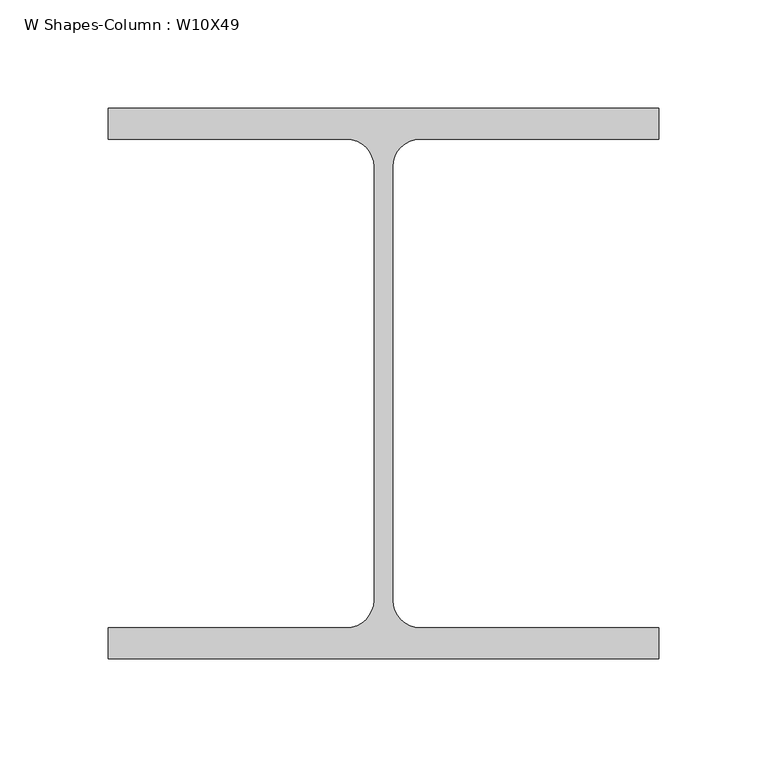
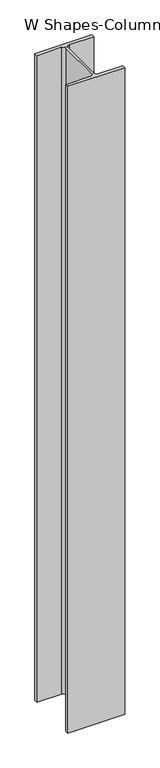
"""IFC4 building model written with IfcOpenShell, lengths in millimetres: column geometry, W Shapes-Column : W10X49."""

from ifc_helpers import new_model, si_unit, point, frame, frame_2d, origin, place, context, project, spatial, polyline, circle_curve, trimmed, segment, composite_curve, outline, extrude, source, transform, mapped, element, save


def w_shapes_column_w10x49_c7b378f5(model_context):
    return source(origin(), model_context, "Body", "SweptSolid", [
        extrude(outline(composite_curve([segment(polyline([(127.0, 127.0), (127.0, 112.776), (17.018, 112.776)]), True, "CONTINUOUS"), segment(trimmed(circle_curve(frame_2d((17.018, 100.076)), 12.7), [point((17.018, 112.776))], [point((4.318, 100.076))], True, "CARTESIAN"), True, "CONTINUOUS"), segment(polyline([(4.318, 100.076), (4.318, -100.076)]), True, "CONTINUOUS"), segment(trimmed(circle_curve(frame_2d((17.018, -100.076)), 12.7), [point((4.318, -100.076))], [point((17.018, -112.776))], True, "CARTESIAN"), True, "CONTINUOUS"), segment(polyline([(17.018, -112.776), (127.0, -112.776), (127.0, -127.0), (-127.0, -127.0), (-127.0, -112.776), (-17.018, -112.776)]), True, "CONTINUOUS"), segment(trimmed(circle_curve(frame_2d((-17.018, -100.076)), 12.7), [point((-17.018, -112.776))], [point((-4.318, -100.076))], True, "CARTESIAN"), True, "CONTINUOUS"), segment(polyline([(-4.318, -100.076), (-4.318, 100.076)]), True, "CONTINUOUS"), segment(trimmed(circle_curve(frame_2d((-17.018, 100.076)), 12.7), [point((-4.318, 100.076))], [point((-17.018, 112.776))], True, "CARTESIAN"), True, "CONTINUOUS"), segment(polyline([(-17.018, 112.776), (-127.0, 112.776), (-127.0, 127.0), (127.0, 127.0)]), True, "CONTINUOUS")], self_intersect=False)), frame((0.0, 0.0, 6096.0), z_axis=(0.0, 0.0, 1.0), x_axis=(1.0, 0.0, 0.0)), (0.0, 0.0, 1.0), 3048.0),
    ])


if __name__ == "__main__":
    model = new_model("IFC4")
    model_context = context("Model", 3, world=origin())
    ifc_project = project(units=[si_unit("LENGTHUNIT", "METRE", prefix="MILLI")], contexts=[model_context])
    site = spatial("IfcSite", under=ifc_project)
    building = spatial("IfcBuilding", under=site)
    placement = place(None, origin())
    w_shapes_column_w10x49_shape = w_shapes_column_w10x49_c7b378f5(model_context)
    element("IfcColumn", 1, ObjectType="W Shapes-Column : W10X49", at=placement, inside=building, context=model_context, shape_type="MappedRepresentation", body=[
        mapped(w_shapes_column_w10x49_shape, transform((0.0, 0.0, 0.0), x_axis=(1.0, 0.0, 0.0), y_axis=(0.0, 1.0, 0.0), z_axis=(0.0, 0.0, 1.0))),
    ])
    save(model, "model.ifc")

# Revit data of these elements
# Type "W Shapes-Column : W10X49"
#   Section Name Key = "W10x49"
#   Assembly Code = "B10"
#   Width = 10.000"
#   Web Thickness = 0.340"
#   Web Fillet = 0.500"
#   Warping Constant = 2070.00 in⁶
#   Torsional Moment of Inertia = 1.39 in⁴
#   Section Area = 14.40 in²
#   Plastic Modulus weak axis = 28.30 in³
#   Plastic Modulus strong axis = 60.40 in³
#   Perimeter = 58.50 ft²/ft
#   Nominal Weight = 49.00 lbf/ft
#   Moment of Inertia weak axis = 93.40 in⁴
#   Moment of Inertia strong axis = 272.00 in⁴
#   Height = 10.000"
#   Flange Thickness = 0.560"
#   Elastic Modulus weak axis = 18.70 in³
#   Elastic Modulus strong axis = 54.60 in³
#   Centroid Vertical = 5.000"
#   Centroid Horizontal = 5.000"
#   Bolt Spacing = 0' - 5 1/2"
#   Structural Material [instance default] = Steel ASTM A992
#   Principal Axes Angle = 0
# Element 1 (IfcColumn, "W Shapes-Column : W10X49")
#   Materials on its faces: "Steel ASTM A992"
# Materials
#   "Steel ASTM A992": class "Metal", colour RGB 199 199 199, transparency 0, Description = "Structural steel 50ksi", Cost = 0
